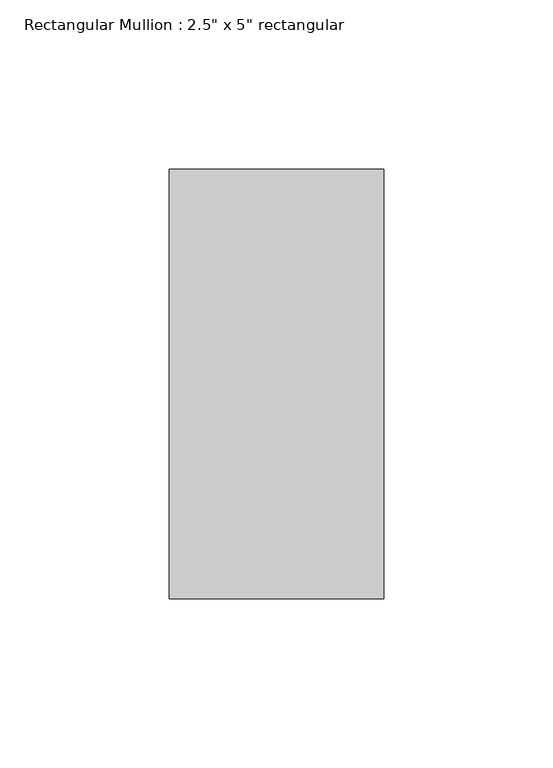
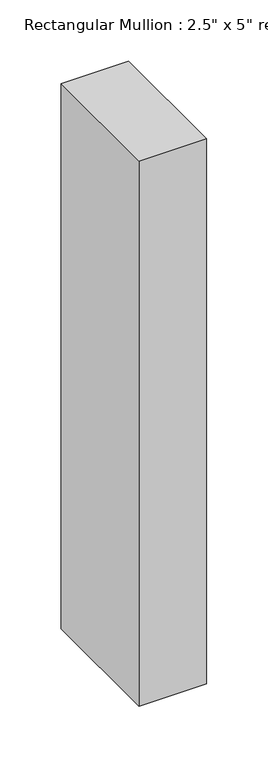
"""IFC4 building model written with IfcOpenShell, lengths in millimetres: member geometry."""

from ifc_helpers import new_model, si_unit, frame, origin, place, context, project, spatial, polyline, outline, extrude, source, transform, mapped, element, save


def member_668e8779(model_context):
    return source(origin(), model_context, "Body", "SweptSolid", [
        extrude(outline(polyline([(0.0, 63.5), (0.0, -63.5), (-63.5, -63.5), (-63.5, 63.5), (0.0, 63.5)])), frame((0.0, 0.0, -542.516556), z_axis=(0.0, 0.0, 1.0), x_axis=(1.0, 0.0, 0.0)), (0.0, 0.0, 1.0), 542.516556),
    ])


if __name__ == "__main__":
    model = new_model("IFC4")
    model_context = context("Model", 3, world=origin())
    ifc_project = project(units=[si_unit("LENGTHUNIT", "METRE", prefix="MILLI")], contexts=[model_context])
    site = spatial("IfcSite", under=ifc_project)
    building = spatial("IfcBuilding", under=site)
    placement = place(None, origin())
    member_shape = member_668e8779(model_context)
    element("IfcMember", 1, ObjectType="Rectangular Mullion : 2.5\" x 5\" rectangular", at=placement, inside=building, context=model_context, shape_type="MappedRepresentation", body=[
        mapped(member_shape, transform((0.0, 0.0, 0.0), x_axis=(1.0, 0.0, 0.0), y_axis=(0.0, 1.0, 0.0), z_axis=(0.0, 0.0, 1.0))),
    ])
    save(model, "model.ifc")

# Revit data of these elements
# Type "Rectangular Mullion : 2.5\" x 5\" rectangular"
#   built-in parameter 1007304 = 0.416667 (stored number, unit not read)
#   built-in parameter 1007301 = 0.104167 (stored number, unit not read)
#   built-in parameter 1007300 = 0.104167 (stored number, unit not read)
# Element 1 (IfcMember, "Rectangular Mullion : 2.5\" x 5\" rectangular")
#   Materials on its faces: "Aluminum"
# Materials
#   "Aluminum": class "Metal", colour RGB 247 247 247, transparency 0, Description = "Aluminum 6061", Cost = 0
